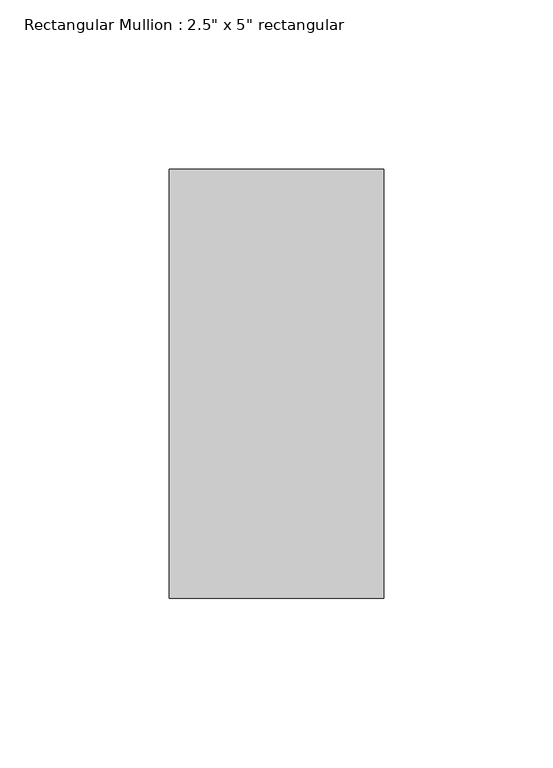
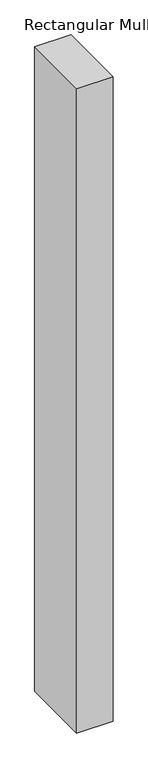
"""IFC4 building model written with IfcOpenShell, lengths in millimetres: member geometry."""

from ifc_helpers import new_model, si_unit, frame, origin, place, context, project, spatial, polyline, outline, extrude, source, transform, mapped, element, save


def member_1434c356(model_context):
    return source(origin(), model_context, "Body", "SweptSolid", [
        extrude(outline(polyline([(0.0, 63.5), (0.0, -63.5), (-63.5, -63.5), (-63.5, 63.5), (0.0, 63.5)])), frame((0.0, 0.0, -1187.2492225), z_axis=(0.0, 0.0, 1.0), x_axis=(1.0, 0.0, 0.0)), (0.0, 0.0, 1.0), 1187.2492225),
    ])


if __name__ == "__main__":
    model = new_model("IFC4")
    model_context = context("Model", 3, world=origin())
    ifc_project = project(units=[si_unit("LENGTHUNIT", "METRE", prefix="MILLI")], contexts=[model_context])
    site = spatial("IfcSite", under=ifc_project)
    building = spatial("IfcBuilding", under=site)
    placement = place(None, origin())
    member_shape = member_1434c356(model_context)
    element("IfcMember", 1, ObjectType="Rectangular Mullion : 2.5\" x 5\" rectangular", at=placement, inside=building, context=model_context, shape_type="MappedRepresentation", body=[
        mapped(member_shape, transform((0.0, 0.0, 0.0), x_axis=(1.0, 0.0, 0.0), y_axis=(0.0, 1.0, 0.0), z_axis=(0.0, 0.0, 1.0))),
    ])
    save(model, "model.ifc")

# Revit data of these elements
# Type "Rectangular Mullion : 2.5\" x 5\" rectangular"
#   built-in parameter 1007304 = 0.416667 (stored number, unit not read)
#   built-in parameter 1007301 = 0.104167 (stored number, unit not read)
#   built-in parameter 1007300 = 0.104167 (stored number, unit not read)
# Element 1 (IfcMember, "Rectangular Mullion : 2.5\" x 5\" rectangular")
#   Materials on its faces: "Aluminum"
# Materials
#   "Aluminum": class "Metal", colour RGB 247 247 247, transparency 0, Description = "Aluminum 6061", Cost = 0
